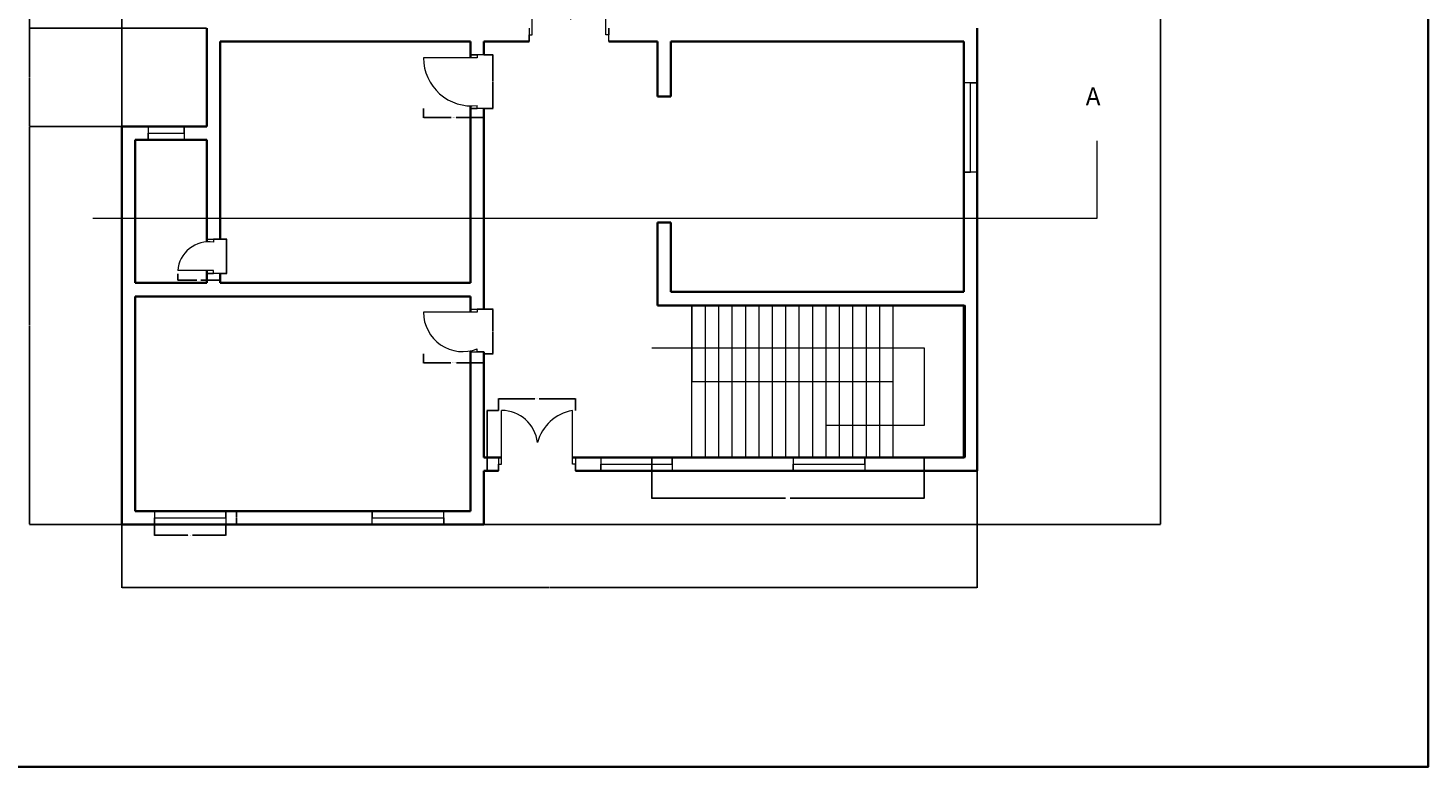
# Model space of a CAD drawing. Units: inches. Extents: x 1824 to 3509, y 619 to 2294.
# Tile 9 of 12: x 2570 to 3509, y 619 to 1115. Entities that reach past the tile are written whole.
import ezdxf

# ---------------------------------------------------------------- set-up
doc = ezdxf.new("R2010")
doc.units = ezdxf.units.IN
for name, color, linetype, lineweight in [('A-ANNO-DIMS', 2, 'Continuous', 18), ('A-ANNO-SYMB', 7, 'Continuous', 18), ('A-ANNO-TTLB', 7, 'Continuous', 35), ('A-DOOR', 3, 'Continuous', 18), ('A-FLOR-STRS', 7, 'Continuous', 18), ('A-GLAZ', 4, 'Continuous', 18), ('A-WALL', 7, 'Continuous', 35)]:
    doc.layers.add(name, color=color, linetype=linetype, lineweight=lineweight)
doc.styles.get("Standard").update_dxf_attribs({"font": 'arial.ttf'})
doc.dimstyles.get("Standard").update_dxf_attribs({"dimtxt": 0.18, "dimasz": 0.18, "dimexe": 0.18, "dimexo": 0.0625, "dimgap": 0.09, "dimtad": 0, "dimtih": 1, "dimtoh": 1, "dimdec": 4, "dimzin": 0, "dimdsep": 46, "dimtxsty": 'Standard', "dimcen": 0.09, "dimadec": 0, "dimazin": 0, "dimtfac": 1, "dimtdec": 4, "dimtofl": 0, "dimtmove": 0, "dimatfit": 3, "dimfxl": 1, "dimtolj": 1, "dimtzin": 0, "dimarcsym": 0})

# ---------------------------------------------------------------- blocks, each defined once
blk = doc.blocks.new('STAIR-RETURN-PLAN')
for p, q in [((26.85, 0), (26.85, 102)), ((26.85, 102), (26.85, 51)), ((35.85, 102), (35.85, 0)), ((44.85, 102), (44.85, 0)), ((53.85, 102), (53.85, 0)), ((62.85, 102), (62.85, 0)), ((71.85, 102), (71.85, 0)), ((80.85, 102), (80.85, 0)), ((89.85, 102), (89.85, 0)), ((98.85, 102), (98.85, 0)), ((107.85, 102), (107.85, 0)), ((116.85, 102), (116.85, 0)), ((125.85, 102), (125.85, 0)), ((134.85, 102), (134.85, 0)), ((143.85, 102), (143.85, 0)), ((152.85, 102), (152.85, 0)), ((161.85, 102), (161.85, 0)), ((0, 73.44), (182.85, 73.44)), ((182.85, 73.44), (182.85, 21.48)), ((26.85, 51), (161.85, 51)), ((182.85, 21.48), (116.85, 21.48))]:
    blk.add_line(p, q)
blk = doc.blocks.new('DOOR-LOUNGE-PAIR')
for p, q in [((2, 4.5), (2, 40.5)), ((51.41, 4.5), (51.41, 40.5)), ((27.9, 14.63), (27.9, 18.05)), ((0, 9), (0, 0)), ((0, 0), (0, 4.5)), ((0, 4.5), (2, 4.5)), ((53.41, 4.5), (51.41, 4.5)), ((53.41, 0), (53.41, 9)), ((53.41, 9), (53.41, 4.5)), ((53.41, 4.5), (53.41, 4.5))]:
    blk.add_line(p, q)
for centre, radius, start, end in [((-0.78, 11.81), 28.82, 5.60143, 84.45665), ((54.5, 13.67), 27.01, 96.57316, 173.88946)]:
    blk.add_arc(centre, radius, start, end)
blk = doc.blocks.new('DOOR-BED-FRONT-36')
for p, q in [((36, 33.97), (0, 33.97)), ((40.5, 35.97), (31.5, 35.97)), ((31.5, 35.97), (36, 35.97)), ((36, 35.97), (36, 33.97)), ((40.5, 35.97), (40.5, 35.97)), ((40.5, 0), (31.5, 0)), ((31.5, 0), (31.5, 0)), ((31.5, 0), (36, 0)), ((36, 0), (36, 2))]:
    blk.add_line(p, q)
blk.add_arc((32.19, 33.97), 32.19, 180, 276.79209)
blk = doc.blocks.new('DOOR-BATH-FRONT-24')
for p, q in [((19.5, 23.21), (28.5, 23.21)), ((28.5, 23.21), (24, 23.21)), ((24, 23.21), (24, 21.21)), ((28.5, 23.21), (28.5, 23.21)), ((24, 2), (0, 2)), ((24, 0), (24, 2)), ((28.5, 0), (19.5, 0)), ((19.5, 0), (24, 0)), ((24, 0), (24, 0))]:
    blk.add_line(p, q)
blk.add_arc((21.09, 0.25), 21.16, 82.09424, 175.25862)
blk = doc.blocks.new('DOOR-DRAWING-36')
for p, q in [((31.55, 28.63), (37.79, 28.63)), ((40.55, 28.63), (36, 28.63)), ((36, 28.63), (36, 26.63)), ((37.79, 28.63), (40.55, 28.63)), ((36, 26.63), (0, 26.63)), ((36.05, 0), (36.05, 2)), ((31.55, 0), (40.55, 0)), ((40.55, 0), (36.05, 0))]:
    blk.add_line(p, q)
blk.add_arc((26.44, 26.63), 26.44, 180, 291.32239)
blk = doc.blocks.new('DOOR-ENTRY-PAIR')
for p, q in [((2, 4.5), (2, 40.5)), ((49.54, 4.5), (49.54, 40.5)), ((0, 9), (0, 0)), ((0, 0), (0, 4.5)), ((0, 4.5), (2, 4.5)), ((51.54, 4.5), (49.54, 4.5)), ((51.54, 9), (51.54, 0)), ((51.54, 0), (51.54, 4.5))]:
    blk.add_line(p, q)
for centre, radius, start, end in [((2, 16.28), 24.22, 6.41309, 90), ((54.84, 11.16), 29.82, 100.24251, 164.77967)]:
    blk.add_arc(centre, radius, start, end)
blk = doc.blocks.new('WIN-24')
for p, q in [((0, 0), (0, 9)), ((0, 9), (0, 4.5)), ((0, 4.5), (24, 4.5)), ((24, 0), (24, 9)), ((24, 4.5), (24, 0))]:
    blk.add_line(p, q)
blk = doc.blocks.new('WIN-48')
for p, q in [((0, 9), (0, 0)), ((0, 0), (0, 4.5)), ((0, 4.5), (48, 4.5)), ((48, 4.5), (48, 9)), ((48, 9), (48, 0))]:
    blk.add_line(p, q)
blk = doc.blocks.new('WIN-60')
for p, q in [((0, 9), (0, 0)), ((0, 0), (0, 4.5)), ((0, 4.5), (60, 4.5)), ((60, 4.5), (60, 9)), ((60, 9), (60, 0))]:
    blk.add_line(p, q)
blk = doc.blocks.new('*D34')
at = {"layer": 'A-ANNO-DIMS', "color": 0, "lineweight": -2, "transparency": 16777216}
for p, q in [((2654.59, 782.04), (2654.59, 774.72)), ((2702.59, 782.04), (2702.59, 774.72)), ((2654.77, 774.9), (2677.01, 774.9)), ((2702.41, 774.9), (2680.17, 774.9))]:
    blk.add_line(p, q, dxfattribs=at)
at = {"layer": 'A-ANNO-DIMS', "color": 0, "transparency": 16777216}
for points in [[(2654.77, 774.93), (2654.77, 774.87), (2654.59, 774.9)], [(2702.41, 774.93), (2702.41, 774.87), (2702.59, 774.9)]]:
    blk.add_solid(points, dxfattribs=at)
at = {"layer": 'Defpoints', "color": 0, "transparency": 16777216}
for p in [(2654.59, 782.1), (2702.59, 782.1), (2702.59, 774.9)]:
    blk.add_point(p, dxfattribs=at)
at = {"layer": 'A-ANNO-DIMS', "color": 0, "transparency": 16777216, "insert": (2678.59, 774.9), "char_height": 0.18, "attachment_point": 5}
blk.add_mtext('\\A1;FRONT WINDOW 48 TYP.', dxfattribs=at)
blk = doc.blocks.new('*D35')
at = {"layer": 'A-ANNO-DIMS', "color": 0, "lineweight": -2, "transparency": 16777216}
for p, q in [((2702.65, 791.1), (2709.97, 791.1)), ((2709.79, 790.92), (2709.79, 786.78)), ((2702.65, 782.1), (2709.97, 782.1)), ((2709.79, 782.28), (2709.79, 786.42))]:
    blk.add_line(p, q, dxfattribs=at)
at = {"layer": 'A-ANNO-DIMS', "color": 0, "transparency": 16777216}
for points in [[(2709.76, 790.92), (2709.82, 790.92), (2709.79, 791.1)], [(2709.76, 782.28), (2709.82, 782.28), (2709.79, 782.1)]]:
    blk.add_solid(points, dxfattribs=at)
at = {"layer": 'Defpoints', "color": 0, "transparency": 16777216}
for p in [(2702.59, 791.1), (2709.79, 791.1), (2702.59, 782.1)]:
    blk.add_point(p, dxfattribs=at)
at = {"layer": 'A-ANNO-DIMS', "color": 0, "transparency": 16777216, "insert": (2709.79, 786.6), "char_height": 0.18, "attachment_point": 5}
blk.add_mtext('\\A1;9 TYP.', dxfattribs=at)
blk = doc.blocks.new('*D50')
at = {"layer": 'A-ANNO-DIMS', "color": 0, "lineweight": -2, "transparency": 16777216}
for p, q in [((2988.36, 827.04), (2988.36, 799.49)), ((3171.21, 827.04), (3171.21, 799.49)), ((2988.54, 799.67), (3078.23, 799.67)), ((3171.03, 799.67), (3081.34, 799.67))]:
    blk.add_line(p, q, dxfattribs=at)
at = {"layer": 'A-ANNO-DIMS', "color": 0, "transparency": 16777216}
for points in [[(2988.54, 799.7), (2988.54, 799.64), (2988.36, 799.67)], [(3171.03, 799.7), (3171.03, 799.64), (3171.21, 799.67)]]:
    blk.add_solid(points, dxfattribs=at)
at = {"layer": 'Defpoints', "color": 0, "transparency": 16777216}
for p in [(2988.36, 827.1), (3171.21, 827.1), (3171.21, 799.67)]:
    blk.add_point(p, dxfattribs=at)
at = {"layer": 'A-ANNO-DIMS', "color": 0, "transparency": 16777216, "insert": (3079.78, 799.67), "char_height": 0.18, "attachment_point": 5}
blk.add_mtext('\\A1;RETURN STAIR 183 TYP.', dxfattribs=at)
blk = doc.blocks.new('*D51')
at = {"layer": 'A-ANNO-DIMS', "color": 0, "lineweight": -2, "transparency": 16777216}
for p, q in [((3171.27, 929.1), (3198.81, 929.1)), ((3198.63, 928.92), (3198.63, 878.28)), ((3198.63, 827.28), (3198.63, 877.92)), ((3171.27, 827.1), (3198.81, 827.1))]:
    blk.add_line(p, q, dxfattribs=at)
at = {"layer": 'A-ANNO-DIMS', "color": 0, "transparency": 16777216}
for points in [[(3198.6, 928.92), (3198.66, 928.92), (3198.63, 929.1)], [(3198.6, 827.28), (3198.66, 827.28), (3198.63, 827.1)]]:
    blk.add_solid(points, dxfattribs=at)
at = {"layer": 'Defpoints', "color": 0, "transparency": 16777216}
for p in [(3171.21, 929.1), (3198.63, 929.1), (3171.21, 827.1)]:
    blk.add_point(p, dxfattribs=at)
at = {"layer": 'A-ANNO-DIMS', "color": 0, "transparency": 16777216, "insert": (3198.63, 878.1), "char_height": 0.18, "attachment_point": 5}
blk.add_mtext('\\A1;102 TYP.', dxfattribs=at)
blk = doc.blocks.new('*D76')
at = {"layer": 'A-ANNO-DIMS', "color": 0, "lineweight": -2, "transparency": 16777216}
for p, q in [((2835.23, 1061.02), (2835.23, 1054.83)), ((2835.41, 1055.01), (2853.86, 1055.01)), ((2875.55, 1055.01), (2857.1, 1055.01)), ((2875.73, 1061.02), (2875.73, 1054.83))]:
    blk.add_line(p, q, dxfattribs=at)
at = {"layer": 'A-ANNO-DIMS', "color": 0, "transparency": 16777216}
for points in [[(2835.41, 1055.04), (2835.41, 1054.98), (2835.23, 1055.01)], [(2875.55, 1055.04), (2875.55, 1054.98), (2875.73, 1055.01)]]:
    blk.add_solid(points, dxfattribs=at)
at = {"layer": 'Defpoints', "color": 0, "transparency": 16777216}
for p in [(2835.23, 1061.08), (2875.73, 1061.08), (2875.73, 1055.01)]:
    blk.add_point(p, dxfattribs=at)
at = {"layer": 'A-ANNO-DIMS', "color": 0, "transparency": 16777216, "insert": (2855.48, 1055.01), "char_height": 0.18, "attachment_point": 5}
blk.add_mtext('\\A1;BEDROOM DOOR 41 TYP.', dxfattribs=at)
blk = doc.blocks.new('*D77')
at = {"layer": 'A-ANNO-DIMS', "color": 0, "lineweight": -2, "transparency": 16777216}
for p, q in [((2875.79, 1097.05), (2881.98, 1097.05)), ((2881.8, 1096.87), (2881.8, 1079.25)), ((2881.8, 1061.26), (2881.8, 1078.88)), ((2875.79, 1061.08), (2881.98, 1061.08))]:
    blk.add_line(p, q, dxfattribs=at)
at = {"layer": 'A-ANNO-DIMS', "color": 0, "transparency": 16777216}
for points in [[(2881.77, 1096.87), (2881.83, 1096.87), (2881.8, 1097.05)], [(2881.77, 1061.26), (2881.83, 1061.26), (2881.8, 1061.08)]]:
    blk.add_solid(points, dxfattribs=at)
at = {"layer": 'Defpoints', "color": 0, "transparency": 16777216}
for p in [(2875.73, 1097.05), (2881.8, 1097.05), (2875.73, 1061.08)]:
    blk.add_point(p, dxfattribs=at)
at = {"layer": 'A-ANNO-DIMS', "color": 0, "transparency": 16777216, "insert": (2881.8, 1079.06), "char_height": 0.18, "attachment_point": 5}
blk.add_mtext('\\A1;36 TYP.', dxfattribs=at)
blk = doc.blocks.new('*D78')
at = {"layer": 'A-ANNO-DIMS', "color": 0, "lineweight": -2, "transparency": 16777216}
for p, q in [((2670.23, 950.31), (2670.23, 945.91)), ((2698.73, 950.31), (2698.73, 945.91)), ((2670.41, 946.09), (2683.17, 946.09)), ((2698.55, 946.09), (2685.78, 946.09))]:
    blk.add_line(p, q, dxfattribs=at)
at = {"layer": 'A-ANNO-DIMS', "color": 0, "transparency": 16777216}
for points in [[(2670.41, 946.12), (2670.41, 946.06), (2670.23, 946.09)], [(2698.55, 946.12), (2698.55, 946.06), (2698.73, 946.09)]]:
    blk.add_solid(points, dxfattribs=at)
at = {"layer": 'Defpoints', "color": 0, "transparency": 16777216}
for p in [(2670.23, 950.37), (2698.73, 950.37), (2698.73, 946.09)]:
    blk.add_point(p, dxfattribs=at)
at = {"layer": 'A-ANNO-DIMS', "color": 0, "transparency": 16777216, "insert": (2684.48, 946.09), "char_height": 0.18, "attachment_point": 5}
blk.add_mtext('\\A1;BATH DOOR 29 TYP.', dxfattribs=at)
blk = doc.blocks.new('*D79')
at = {"layer": 'A-ANNO-DIMS', "color": 0, "lineweight": -2, "transparency": 16777216}
for p, q in [((2698.79, 973.58), (2703.18, 973.58)), ((2703, 973.4), (2703, 962.16)), ((2703, 950.55), (2703, 961.79)), ((2698.79, 950.37), (2703.18, 950.37))]:
    blk.add_line(p, q, dxfattribs=at)
at = {"layer": 'A-ANNO-DIMS', "color": 0, "transparency": 16777216}
for points in [[(2702.97, 973.4), (2703.03, 973.4), (2703, 973.58)], [(2702.97, 950.55), (2703.03, 950.55), (2703, 950.37)]]:
    blk.add_solid(points, dxfattribs=at)
at = {"layer": 'Defpoints', "color": 0, "transparency": 16777216}
for p in [(2698.73, 973.58), (2703, 973.58), (2698.73, 950.37)]:
    blk.add_point(p, dxfattribs=at)
at = {"layer": 'A-ANNO-DIMS', "color": 0, "transparency": 16777216, "insert": (2703, 961.97), "char_height": 0.18, "attachment_point": 5}
blk.add_mtext('\\A1;23 TYP.', dxfattribs=at)
blk = doc.blocks.new('*D80')
at = {"layer": 'A-ANNO-DIMS', "color": 0, "lineweight": -2, "transparency": 16777216}
for p, q in [((2835.18, 896.61), (2835.18, 890.41)), ((2875.73, 896.61), (2875.73, 890.41)), ((2835.36, 890.59), (2853.45, 890.59)), ((2875.55, 890.59), (2857.46, 890.59))]:
    blk.add_line(p, q, dxfattribs=at)
at = {"layer": 'A-ANNO-DIMS', "color": 0, "transparency": 16777216}
for points in [[(2835.36, 890.62), (2835.36, 890.56), (2835.18, 890.59)], [(2875.55, 890.62), (2875.55, 890.56), (2875.73, 890.59)]]:
    blk.add_solid(points, dxfattribs=at)
at = {"layer": 'Defpoints', "color": 0, "transparency": 16777216}
for p in [(2835.18, 896.67), (2875.73, 896.67), (2875.73, 890.59)]:
    blk.add_point(p, dxfattribs=at)
at = {"layer": 'A-ANNO-DIMS', "color": 0, "transparency": 16777216, "insert": (2855.45, 890.59), "char_height": 0.18, "attachment_point": 5}
blk.add_mtext('\\A1;DRAWING ROOM DOOR 41 TYP.', dxfattribs=at)
blk = doc.blocks.new('*D81')
at = {"layer": 'A-ANNO-DIMS', "color": 0, "lineweight": -2, "transparency": 16777216}
for p, q in [((2875.79, 926.47), (2881.99, 926.47)), ((2881.81, 926.29), (2881.81, 911.75)), ((2881.81, 896.85), (2881.81, 911.39)), ((2875.79, 896.67), (2881.99, 896.67))]:
    blk.add_line(p, q, dxfattribs=at)
at = {"layer": 'A-ANNO-DIMS', "color": 0, "transparency": 16777216}
for points in [[(2881.78, 926.29), (2881.84, 926.29), (2881.81, 926.47)], [(2881.78, 896.85), (2881.84, 896.85), (2881.81, 896.67)]]:
    blk.add_solid(points, dxfattribs=at)
at = {"layer": 'Defpoints', "color": 0, "transparency": 16777216}
for p in [(2875.73, 926.47), (2881.81, 926.47), (2875.73, 896.67)]:
    blk.add_point(p, dxfattribs=at)
at = {"layer": 'A-ANNO-DIMS', "color": 0, "transparency": 16777216, "insert": (2881.81, 911.57), "char_height": 0.18, "attachment_point": 5}
blk.add_mtext('\\A1;30 TYP.', dxfattribs=at)
blk = doc.blocks.new('*D82')
at = {"layer": 'A-ANNO-DIMS', "color": 0, "lineweight": -2, "transparency": 16777216}
for p, q in [((2885.62, 858.66), (2885.62, 866.51)), ((2885.8, 866.33), (2909.91, 866.33)), ((2936.98, 866.33), (2912.87, 866.33)), ((2937.16, 858.66), (2937.16, 866.51))]:
    blk.add_line(p, q, dxfattribs=at)
at = {"layer": 'A-ANNO-DIMS', "color": 0, "transparency": 16777216}
for points in [[(2885.8, 866.36), (2885.8, 866.3), (2885.62, 866.33)], [(2936.98, 866.36), (2936.98, 866.3), (2937.16, 866.33)]]:
    blk.add_solid(points, dxfattribs=at)
at = {"layer": 'Defpoints', "color": 0, "transparency": 16777216}
for p in [(2937.16, 866.33), (2885.62, 858.6), (2937.16, 858.6)]:
    blk.add_point(p, dxfattribs=at)
at = {"layer": 'A-ANNO-DIMS', "color": 0, "transparency": 16777216, "insert": (2911.39, 866.33), "char_height": 0.18, "attachment_point": 5}
blk.add_mtext('\\A1;ENTRY DOORS 52 TYP.', dxfattribs=at)
blk = doc.blocks.new('*D83')
at = {"layer": 'A-ANNO-DIMS', "color": 0, "lineweight": -2, "transparency": 16777216}
for p, q in [((2885.56, 858.6), (2877.71, 858.6)), ((2877.89, 858.42), (2877.89, 838.53)), ((2877.89, 818.28), (2877.89, 838.17)), ((2885.56, 818.1), (2877.71, 818.1))]:
    blk.add_line(p, q, dxfattribs=at)
at = {"layer": 'A-ANNO-DIMS', "color": 0, "transparency": 16777216}
for points in [[(2877.86, 858.42), (2877.92, 858.42), (2877.89, 858.6)], [(2877.86, 818.28), (2877.92, 818.28), (2877.89, 818.1)]]:
    blk.add_solid(points, dxfattribs=at)
at = {"layer": 'Defpoints', "color": 0, "transparency": 16777216}
for p in [(2877.89, 858.6), (2885.62, 858.6), (2885.62, 818.1)]:
    blk.add_point(p, dxfattribs=at)
at = {"layer": 'A-ANNO-DIMS', "color": 0, "transparency": 16777216, "insert": (2877.89, 838.35), "char_height": 0.18, "attachment_point": 5}
blk.add_mtext('\\A1;41 TYP.', dxfattribs=at)
blk = doc.blocks.new('*D103')
at = {"layer": 'A-ANNO-DIMS', "color": 0, "lineweight": -2, "transparency": 16777216}
for p, q in [((3206.73, 818.04), (3206.73, 739.57)), ((2632.73, 782.04), (2632.73, 739.57)), ((2632.91, 739.75), (2919.44, 739.75)), ((3206.55, 739.75), (2920.02, 739.75))]:
    blk.add_line(p, q, dxfattribs=at)
at = {"layer": 'A-ANNO-DIMS', "color": 0, "transparency": 16777216}
for points in [[(2632.91, 739.78), (2632.91, 739.72), (2632.73, 739.75)], [(3206.55, 739.78), (3206.55, 739.72), (3206.73, 739.75)]]:
    blk.add_solid(points, dxfattribs=at)
at = {"layer": 'Defpoints', "color": 0, "transparency": 16777216}
for p in [(3206.73, 818.1), (2632.73, 782.1), (3206.73, 739.75)]:
    blk.add_point(p, dxfattribs=at)
at = {"layer": 'A-ANNO-DIMS', "color": 0, "transparency": 16777216, "insert": (2919.73, 739.75), "char_height": 0.18, "attachment_point": 5}
blk.add_mtext('\\A1;574', dxfattribs=at)
blk = doc.blocks.new('*D104')
at = {"layer": 'A-ANNO-DIMS', "color": 0, "lineweight": -2, "transparency": 16777216}
for p, q in [((3206.79, 1622.1), (3329.93, 1622.1)), ((3329.75, 1621.92), (3329.75, 1202.28)), ((3329.75, 782.28), (3329.75, 1201.92)), ((2875.79, 782.1), (3329.93, 782.1))]:
    blk.add_line(p, q, dxfattribs=at)
at = {"layer": 'A-ANNO-DIMS', "color": 0, "transparency": 16777216}
for points in [[(3329.72, 1621.92), (3329.78, 1621.92), (3329.75, 1622.1)], [(3329.72, 782.28), (3329.78, 782.28), (3329.75, 782.1)]]:
    blk.add_solid(points, dxfattribs=at)
at = {"layer": 'Defpoints', "color": 0, "transparency": 16777216}
for p in [(3206.73, 1622.1), (3329.75, 1622.1), (2875.73, 782.1)]:
    blk.add_point(p, dxfattribs=at)
at = {"layer": 'A-ANNO-DIMS', "color": 0, "transparency": 16777216, "insert": (3329.75, 1202.1), "char_height": 0.18, "attachment_point": 5}
blk.add_mtext('\\A1;840', dxfattribs=at)
blk = doc.blocks.new('*D105')
at = {"layer": 'A-ANNO-DIMS', "color": 0, "lineweight": -2, "transparency": 16777216}
for p, q in [((2632.67, 1049.1), (2570.72, 1049.1)), ((2570.9, 1048.92), (2570.9, 915.78)), ((2570.9, 782.28), (2570.9, 915.42)), ((2632.67, 782.1), (2570.72, 782.1))]:
    blk.add_line(p, q, dxfattribs=at)
at = {"layer": 'A-ANNO-DIMS', "color": 0, "transparency": 16777216}
for points in [[(2570.87, 1048.92), (2570.93, 1048.92), (2570.9, 1049.1)], [(2570.87, 782.28), (2570.93, 782.28), (2570.9, 782.1)]]:
    blk.add_solid(points, dxfattribs=at)
at = {"layer": 'Defpoints', "color": 0, "transparency": 16777216}
for p in [(2570.9, 1049.1), (2632.73, 1049.1), (2632.73, 782.1)]:
    blk.add_point(p, dxfattribs=at)
at = {"layer": 'A-ANNO-DIMS', "color": 0, "transparency": 16777216, "insert": (2570.9, 915.6), "char_height": 0.18, "attachment_point": 5}
blk.add_mtext('\\A1;267', dxfattribs=at)
blk = doc.blocks.new('*D106')
at = {"layer": 'A-ANNO-DIMS', "color": 0, "lineweight": -2, "transparency": 16777216}
for p, q in [((2689.67, 1115.1), (2570.72, 1115.1)), ((2570.9, 1114.92), (2570.9, 1082.28)), ((2570.9, 1049.28), (2570.9, 1081.92)), ((2632.67, 1049.1), (2570.72, 1049.1))]:
    blk.add_line(p, q, dxfattribs=at)
at = {"layer": 'A-ANNO-DIMS', "color": 0, "transparency": 16777216}
for points in [[(2570.87, 1114.92), (2570.93, 1114.92), (2570.9, 1115.1)], [(2570.87, 1049.28), (2570.93, 1049.28), (2570.9, 1049.1)]]:
    blk.add_solid(points, dxfattribs=at)
at = {"layer": 'Defpoints', "color": 0, "transparency": 16777216}
for p in [(2570.9, 1115.1), (2689.73, 1115.1), (2632.73, 1049.1)]:
    blk.add_point(p, dxfattribs=at)
at = {"layer": 'A-ANNO-DIMS', "color": 0, "transparency": 16777216, "insert": (2570.9, 1082.1), "char_height": 0.18, "attachment_point": 5}
blk.add_mtext('\\A1;66', dxfattribs=at)
blk = doc.blocks.new('*D107')
at = {"layer": 'A-ANNO-DIMS', "color": 0, "lineweight": -2, "transparency": 16777216}
for p, q in [((2712.28, 1188.68), (2570.72, 1188.68)), ((2570.9, 1188.5), (2570.9, 1152.07)), ((2570.9, 1115.28), (2570.9, 1151.71)), ((2689.67, 1115.1), (2570.72, 1115.1))]:
    blk.add_line(p, q, dxfattribs=at)
at = {"layer": 'A-ANNO-DIMS', "color": 0, "transparency": 16777216}
for points in [[(2570.87, 1188.5), (2570.93, 1188.5), (2570.9, 1188.68)], [(2570.87, 1115.28), (2570.93, 1115.28), (2570.9, 1115.1)]]:
    blk.add_solid(points, dxfattribs=at)
at = {"layer": 'Defpoints', "color": 0, "transparency": 16777216}
for p in [(2570.9, 1188.68), (2712.34, 1188.68), (2689.73, 1115.1)]:
    blk.add_point(p, dxfattribs=at)
at = {"layer": 'A-ANNO-DIMS', "color": 0, "transparency": 16777216, "insert": (2570.9, 1151.89), "char_height": 0.18, "attachment_point": 5}
blk.add_mtext('\\A1;73.58', dxfattribs=at)
blk = doc.blocks.new('*D111')
at = {"layer": 'A-ANNO-DIMS', "color": 0, "lineweight": -2, "transparency": 16777216}
for p, q in [((2632.73, 1049.16), (2632.73, 1664.63)), ((2632.91, 1664.45), (2661.01, 1664.45)), ((2689.55, 1664.45), (2661.45, 1664.45)), ((2689.73, 1283.16), (2689.73, 1664.63))]:
    blk.add_line(p, q, dxfattribs=at)
at = {"layer": 'A-ANNO-DIMS', "color": 0, "transparency": 16777216}
for points in [[(2632.91, 1664.48), (2632.91, 1664.42), (2632.73, 1664.45)], [(2689.55, 1664.48), (2689.55, 1664.42), (2689.73, 1664.45)]]:
    blk.add_solid(points, dxfattribs=at)
at = {"layer": 'Defpoints', "color": 0, "transparency": 16777216}
for p in [(2632.73, 1664.45), (2689.73, 1283.1), (2632.73, 1049.1)]:
    blk.add_point(p, dxfattribs=at)
at = {"layer": 'A-ANNO-DIMS', "color": 0, "transparency": 16777216, "insert": (2661.23, 1664.45), "char_height": 0.18, "attachment_point": 5}
blk.add_mtext('\\A1;57', dxfattribs=at)

msp = doc.modelspace()

# ---------------------------------------------------------------- linework, layer by layer
at = {"layer": 'A-ANNO-SYMB'}
for p, q in [((3287.4013, 987.6012), (3287.4013, 1039.416)), ((2613.2484, 987.6012), (3287.4013, 987.6012))]:
    msp.add_line(p, q, dxfattribs=at)
at = {"layer": 'A-ANNO-TTLB'}
msp.add_lwpolyline([(1824.0608, 2293.6614), (3509.3484, 2293.6614), (3509.3484, 619.4665), (1824.0608, 619.4665)], close=True, dxfattribs=at)
at = {"layer": 'A-GLAZ'}
for p, q in [((3083.2961, 827.1012), (3083.2961, 827.1012)), ((2800.7494, 791.1012), (2800.7494, 791.1012))]:
    msp.add_line(p, q, dxfattribs=at)
at = {"layer": 'A-WALL'}
for p, q in [((2689.7282, 1115.1012), (2689.7282, 1049.1012)), ((3206.7282, 1115.1012), (3206.7282, 818.1012)), ((2698.7282, 1106.1012), (2698.7282, 973.58)), ((2698.7282, 1106.1012), (2866.7282, 1106.1012)), ((2866.7282, 1106.1012), (2866.7282, 1095.0468)), ((2875.7282, 1106.1012), (2875.7282, 1097.0468)), ((2906.0784, 1106.1012), (2875.7282, 1106.1012)), ((2992.2282, 1106.1012), (2959.4861, 1106.1012)), ((2992.2282, 1106.1012), (2992.2282, 1069.0655)), ((3001.2282, 1106.1012), (3001.2282, 1069.0655)), ((3197.7282, 1106.1012), (3001.2282, 1106.1012)), ((3001.2282, 1106.1012), (3001.2282, 1069.0655)), ((3040.7282, 1106.1012), (3197.7282, 1106.1012)), ((3197.7282, 1106.1012), (3197.7282, 938.1012)), ((2866.7282, 1062.8616), (2866.7282, 944.1012)), ((3001.2282, 1069.0655), (2992.2282, 1069.0655)), ((3001.2282, 1069.0655), (3001.2282, 1069.0655)), ((2875.7282, 1061.08), (2875.7282, 926.4727)), ((2632.7282, 1040.1012), (2632.7282, 1049.1012)), ((2632.7282, 1049.1012), (2689.7282, 1049.1012)), ((2632.7282, 935.1012), (2632.7282, 1040.1012)), ((2650.7282, 1040.1012), (2641.7282, 1040.1012)), ((2641.7282, 1040.1012), (2641.7282, 944.1012)), ((2689.7282, 1040.1012), (2650.7282, 1040.1012)), ((2689.7282, 1040.1012), (2689.7282, 971.7214)), ((2698.7282, 973.58), (2698.7282, 1040.1012)), ((2992.2282, 984.6189), (2992.2282, 929.1012)), ((3001.2282, 984.6189), (2992.2282, 984.6189)), ((3001.2282, 984.6189), (3001.2282, 938.1012)), ((3001.2282, 984.6189), (3001.2282, 938.1012)), ((2689.7282, 952.3686), (2689.7282, 944.1012)), ((2698.7282, 950.3686), (2698.7282, 944.1012)), ((2698.7282, 944.1012), (2698.7282, 950.3686)), ((2641.7282, 944.1012), (2689.7282, 944.1012)), ((2698.7282, 944.1012), (2866.7282, 944.1012)), ((2632.7282, 935.1012), (2632.7282, 782.1012)), ((2689.7282, 935.1012), (2641.7282, 935.1012)), ((2641.7282, 791.1012), (2641.7282, 935.1012)), ((2689.7282, 935.1012), (2866.7282, 935.1012)), ((2689.7282, 935.1012), (2689.7282, 935.1012)), ((2866.7282, 935.1012), (2866.7282, 924.4727)), ((3001.2282, 938.1012), (3197.7282, 938.1012)), ((3197.7282, 929.1012), (2992.2282, 929.1012)), ((3197.7282, 929.1012), (3197.7282, 827.1012)), ((2866.7282, 898.5364), (2866.7282, 791.1012)), ((2875.7282, 897.8469), (2875.7282, 827.1012)), ((2887.6229, 827.1012), (2875.7282, 827.1012)), ((3197.7282, 827.1012), (2935.1639, 827.1012)), ((2875.7282, 818.1012), (2875.7282, 782.1012)), ((2885.6229, 818.1012), (2875.7282, 818.1012)), ((3206.7282, 818.1012), (2937.1639, 818.1012)), ((2689.7282, 791.1012), (2641.7282, 791.1012)), ((2689.7282, 791.1012), (2866.7282, 791.1012)), ((2641.7282, 782.1012), (2632.7282, 782.1012)), ((2632.7282, 782.1012), (2641.7282, 782.1012)), ((2689.7282, 782.1012), (2641.7282, 782.1012)), ((2689.7282, 782.1012), (2875.7282, 782.1012))]:
    msp.add_line(p, q, dxfattribs=at)

# ---------------------------------------------------------------- block references
at = {"layer": 'A-DOOR'}
for name, p in [('DOOR-LOUNGE-PAIR', (2906.0783, 1106.101)), ('DOOR-BED-FRONT-36', (2835.2283, 1061.08)), ('DOOR-BATH-FRONT-24', (2670.2283, 950.369)), ('DOOR-DRAWING-36', (2835.1803, 897.847)), ('DOOR-ENTRY-PAIR', (2885.6233, 818.101))]:
    msp.add_blockref(name, p, dxfattribs=at)
at = {"layer": 'A-FLOR-STRS'}
msp.add_blockref('STAIR-RETURN-PLAN', (2988.3603, 827.101), dxfattribs=at)
at = {"layer": 'A-GLAZ', "extrusion": (0, 0, -1), "zscale": -1}
for name, p, rotation in [('WIN-60', (-3197.728, 1018.336), 90), ('WIN-24', (-2650.4997, 1049.1013), 180), ('WIN-48', (-2800.7496, 791.1013), 180)]:
    msp.add_blockref(name, p, dxfattribs=dict(at, rotation=rotation))
at = {"layer": 'A-GLAZ'}
for p in [(2954.1233, 818.101), (3083.2963, 818.101), (2654.5917, 782.101)]:
    msp.add_blockref('WIN-48', p, dxfattribs=at)

# ---------------------------------------------------------------- texts
at = {"layer": 'A-ANNO-SYMB', "insert": (3279.6189, 1075.2384), "char_height": 12, "attachment_point": 1}
msp.add_mtext_dynamic_manual_height_columns('A', width=30.709491, gutter_width=12.5, heights=[0], dxfattribs=at)

# ---------------------------------------------------------------- dimensions: what is measured, and where the dimension line sits
at = {"layer": 'A-ANNO-DIMS'}
for base, p1, p2, picture, middle in [((2632.7282, 1664.4512), (2689.7282, 1283.1012), (2632.7282, 1049.1012), '*D111', (2661.2282, 1664.4512)), ((3206.7282, 739.7512), (2632.7282, 782.1012), (3206.7282, 818.1012), '*D103', (2919.7282, 739.7512))]:
    dim = msp.add_linear_dim(base=base, p1=p1, p2=p2, dimstyle='Standard', override={"dimdec": 0, "dimlfac": 1, "dimrnd": 0, "dimzin": 0, "dimdsep": 46, "dimlunit": 2}, dxfattribs=at)
    dim.commit()
    dim.dimension.update_dxf_attribs({"geometry": picture, "text_midpoint": middle})
for base, p1, p2, override, picture, middle in [((3329.7513, 1622.1012), (2875.7282, 782.1012), (3206.7282, 1622.1012), {"dimdec": 0, "dimlfac": 1, "dimrnd": 0, "dimzin": 0, "dimdsep": 46, "dimlunit": 2}, '*D104', (3329.7513, 1202.1012)), ((2570.8984, 1188.6773), (2689.7282, 1115.1012), (2712.3386, 1188.6773), {"dimdec": 2, "dimlfac": 1, "dimrnd": 0, "dimzin": 0, "dimdsep": 46, "dimlunit": 2}, '*D107', (2570.8984, 1151.8892)), ((2570.8984, 1115.1012), (2632.7282, 1049.1012), (2689.7282, 1115.1012), {"dimdec": 0, "dimlfac": 1, "dimrnd": 0, "dimzin": 0, "dimdsep": 46, "dimlunit": 2}, '*D106', (2570.8984, 1082.1012)), ((2570.8984, 1049.1012), (2632.7282, 782.1012), (2632.7282, 1049.1012), {"dimdec": 0, "dimlfac": 1, "dimrnd": 0, "dimzin": 0, "dimdsep": 46, "dimlunit": 2}, '*D105', (2570.8984, 915.6012))]:
    dim = msp.add_linear_dim(base=base, p1=p1, p2=p2, angle=90, dimstyle='Standard', override=override, dxfattribs=at)
    dim.commit()
    dim.dimension.update_dxf_attribs({"geometry": picture, "text_midpoint": middle})
for base, p1, p2, picture, middle in [((2881.8032, 1097.0468), (2875.7282, 1061.08), (2875.7282, 1097.0468), '*D77', (2881.8032, 1079.0634)), ((2703.0032, 973.58), (2698.7282, 950.3686), (2698.7282, 973.58), '*D79', (2703.0032, 961.9743)), ((2881.8103, 926.4727), (2875.7282, 896.6716), (2875.7282, 926.4727), '*D81', (2881.8103, 911.5721)), ((3198.6341, 929.1012), (3171.207, 827.1012), (3171.207, 929.1012), '*D51', (3198.6341, 878.1012)), ((2877.8917343146, 858.6011662656), (2885.622891641, 818.1011662656), (2885.622891641, 858.6011662656), '*D83', (2877.8917343146, 838.3511662656)), ((2709.7915, 791.1012), (2702.5915, 782.1012), (2702.5915, 791.1012), '*D35', (2709.7915, 786.6012))]:
    dim = msp.add_linear_dim(base=base, p1=p1, p2=p2, angle=90, text='<> TYP.', dimstyle='Standard', override={"dimdec": 0, "dimlfac": 1, "dimrnd": 0, "dimzin": 0, "dimdsep": 46, "dimlunit": 2}, dxfattribs=at)
    dim.commit()
    dim.dimension.update_dxf_attribs({"geometry": picture, "text_midpoint": middle})
for base, p1, p2, text, picture, middle in [((2875.7282102324, 1055.0050334602), (2835.2282102324, 1061.0800334602), (2875.7282102324, 1061.0800334602), 'BEDROOM DOOR <> TYP.', '*D76', (2855.4782102324, 1055.0050334602)), ((2698.7282102324, 946.0935881496), (2670.2282102324, 950.3685881496), (2698.7282102324, 950.3685881496), 'BATH DOOR <> TYP.', '*D78', (2684.4782102324, 946.0935881496)), ((2875.7282, 890.5894), (2835.1807, 896.6716), (2875.7282, 896.6716), 'DRAWING ROOM DOOR <> TYP.', '*D80', (2855.4544, 890.5894)), ((2937.1639, 866.3323), (2885.6229, 858.6012), (2937.1639, 858.6012), 'ENTRY DOORS <> TYP.', '*D82', (2911.3934, 866.3323)), ((3171.207, 799.6741), (2988.3601, 827.1012), (3171.207, 827.1012), 'RETURN STAIR <> TYP.', '*D50', (3079.7835, 799.6741)), ((2702.5915, 774.9012), (2654.5915, 782.1012), (2702.5915, 782.1012), 'FRONT WINDOW <> TYP.', '*D34', (2678.5915, 774.9012))]:
    dim = msp.add_linear_dim(base=base, p1=p1, p2=p2, text=text, dimstyle='Standard', override={"dimdec": 0, "dimlfac": 1, "dimrnd": 0, "dimzin": 0, "dimdsep": 46, "dimlunit": 2}, dxfattribs=at)
    dim.commit()
    dim.dimension.update_dxf_attribs({"geometry": picture, "text_midpoint": middle})

doc.saveas('drawing.dxf')
